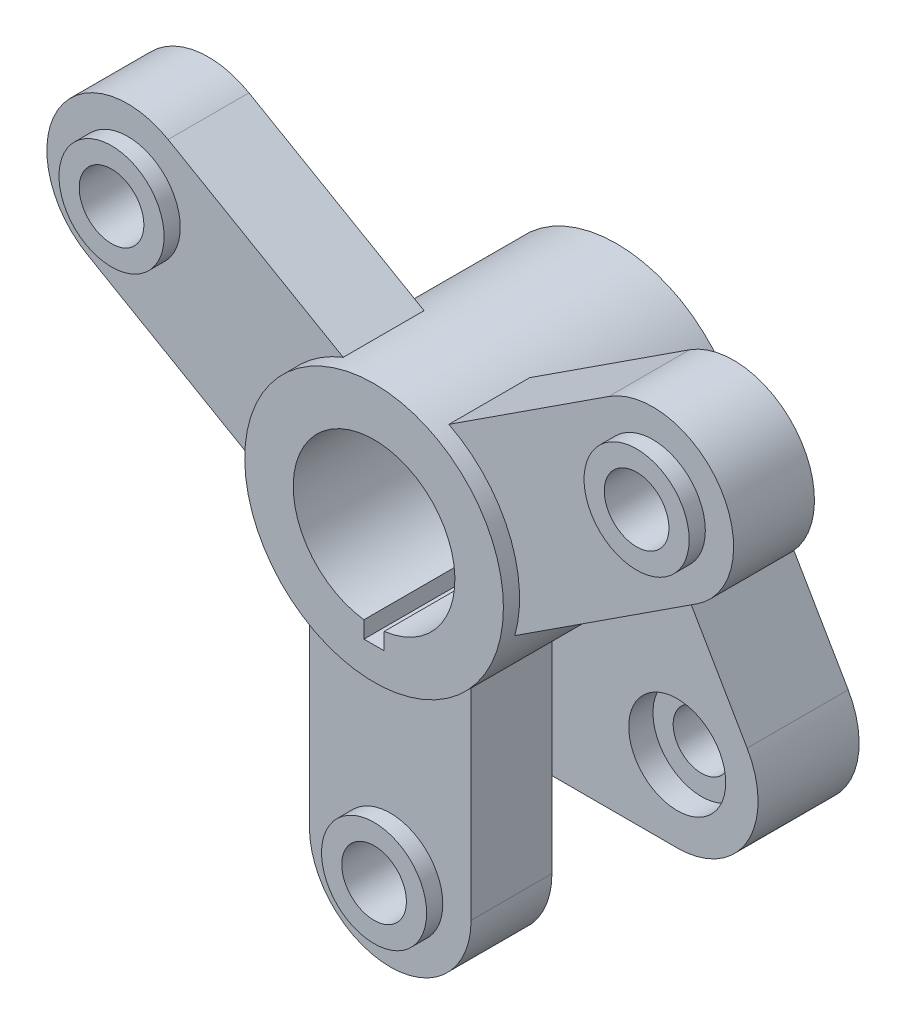
ISO-10303-21;
HEADER;
FILE_DESCRIPTION(('STEP AP214'),'2;1');
FILE_NAME('part.step','',(''),(''),'','','');
FILE_SCHEMA(('AUTOMOTIVE_DESIGN { 1 0 10303 214 1 1 1 1 }'));
ENDSEC;
DATA;
#1=APPLICATION_CONTEXT('core data for automotive mechanical design processes');
#2=APPLICATION_PROTOCOL_DEFINITION('international standard','automotive_design',2000,#1);
#3=PRODUCT_CONTEXT('',#1,'mechanical');
#4=PRODUCT('Part','Part','',(#3));
#5=PRODUCT_RELATED_PRODUCT_CATEGORY('part','',(#4));
#6=PRODUCT_DEFINITION_FORMATION('','',#4);
#7=PRODUCT_DEFINITION_CONTEXT('part definition',#1,'design');
#8=PRODUCT_DEFINITION('design','',#6,#7);
#9=PRODUCT_DEFINITION_SHAPE('','',#8);
#10=(LENGTH_UNIT() NAMED_UNIT(*) SI_UNIT(.MILLI.,.METRE.));
#11=(NAMED_UNIT(*) PLANE_ANGLE_UNIT() SI_UNIT($,.RADIAN.));
#12=(NAMED_UNIT(*) SI_UNIT($,.STERADIAN.) SOLID_ANGLE_UNIT());
#13=UNCERTAINTY_MEASURE_WITH_UNIT(LENGTH_MEASURE(1.E-05),#10,'distance_accuracy_value','');
#14=(GEOMETRIC_REPRESENTATION_CONTEXT(3) GLOBAL_UNCERTAINTY_ASSIGNED_CONTEXT((#13)) GLOBAL_UNIT_ASSIGNED_CONTEXT((#10,
#11,#12)) REPRESENTATION_CONTEXT('',''));
#15=CARTESIAN_POINT('',(0.,0.,0.));
#16=DIRECTION('',(0.,0.,1.));
#17=DIRECTION('',(1.,0.,0.));
#18=AXIS2_PLACEMENT_3D('',#15,#16,#17);
#19=CARTESIAN_POINT('',(0.,0.,56.));
#20=DIRECTION('',(0.,0.,1.));
#21=DIRECTION('',(1.,0.,0.));
#22=AXIS2_PLACEMENT_3D('',#19,#20,#21);
#23=PLANE('',#22);
#24=CARTESIAN_POINT('',(-64.9519052838331,37.4999999999997,56.));
#25=DIRECTION('',(0.,0.,1.));
#26=DIRECTION('',(1.,0.,0.));
#27=AXIS2_PLACEMENT_3D('',#24,#25,#26);
#28=CIRCLE('',#27,13.);
#29=CARTESIAN_POINT('',(-51.9519052838331,37.4999999999997,56.));
#30=VERTEX_POINT('',#29);
#31=EDGE_CURVE('E421',#30,#30,#28,.T.);
#32=ORIENTED_EDGE('',*,*,#31,.F.);
#33=EDGE_LOOP('',(#32));
#34=FACE_BOUND('',#33,.T.);
#35=CARTESIAN_POINT('',(0.,0.,56.));
#36=DIRECTION('',(0.,0.,1.));
#37=DIRECTION('',(1.,0.,0.));
#38=AXIS2_PLACEMENT_3D('',#35,#36,#37);
#39=CIRCLE('',#38,32.);
#40=CARTESIAN_POINT('',(-11.633307652784,29.8105040724855,56.));
#41=VERTEX_POINT('',#40);
#42=CARTESIAN_POINT('',(-31.6333076527839,-4.83051207889206,56.));
#43=VERTEX_POINT('',#42);
#44=EDGE_CURVE('E11',#41,#43,#39,.T.);
#45=ORIENTED_EDGE('',*,*,#44,.F.);
#46=DIRECTION('',(0.866025403784442,-0.499999999999995,0.));
#47=VECTOR('',#46,1.);
#48=CARTESIAN_POINT('',(9.99999999999993,17.3205080756889,56.));
#49=LINE('',#48,#47);
#50=CARTESIAN_POINT('',(-54.9519052838332,54.8205080756885,56.));
#51=VERTEX_POINT('',#50);
#52=EDGE_CURVE('E290',#51,#41,#49,.T.);
#53=ORIENTED_EDGE('',*,*,#52,.F.);
#54=CARTESIAN_POINT('',(-64.9519052838331,37.4999999999997,56.));
#55=DIRECTION('',(0.,0.,1.));
#56=DIRECTION('',(1.,0.,0.));
#57=AXIS2_PLACEMENT_3D('',#54,#55,#56);
#58=CIRCLE('',#57,20.);
#59=CARTESIAN_POINT('',(-74.951905283833,20.1794919243108,56.));
#60=VERTEX_POINT('',#59);
#61=EDGE_CURVE('E309',#51,#60,#58,.T.);
#62=ORIENTED_EDGE('',*,*,#61,.T.);
#63=DIRECTION('',(0.866025403784442,-0.499999999999994,0.));
#64=VECTOR('',#63,1.);
#65=CARTESIAN_POINT('',(-9.99999999999984,-17.3205080756887,56.));
#66=LINE('',#65,#64);
#67=EDGE_CURVE('E299',#60,#43,#66,.T.);
#68=ORIENTED_EDGE('',*,*,#67,.T.);
#69=EDGE_LOOP('',(#45,#53,#62,#68));
#70=FACE_BOUND('',#69,.T.);
#71=ADVANCED_FACE('F50',(#34,#70),#23,.T.);
#72=CARTESIAN_POINT('',(0.,-75.,56.));
#73=DIRECTION('',(0.,0.,1.));
#74=DIRECTION('',(1.,0.,0.));
#75=AXIS2_PLACEMENT_3D('',#72,#73,#74);
#76=CIRCLE('',#75,13.);
#77=CARTESIAN_POINT('',(13.,-75.,56.));
#78=VERTEX_POINT('',#77);
#79=EDGE_CURVE('E414',#78,#78,#76,.T.);
#80=ORIENTED_EDGE('',*,*,#79,.F.);
#81=EDGE_LOOP('',(#80));
#82=FACE_BOUND('',#81,.T.);
#83=CARTESIAN_POINT('',(-20.,-24.9799919935936,56.));
#84=VERTEX_POINT('',#83);
#85=CARTESIAN_POINT('',(20.,-24.9799919935936,56.));
#86=VERTEX_POINT('',#85);
#87=EDGE_CURVE('E57',#84,#86,#39,.T.);
#88=ORIENTED_EDGE('',*,*,#87,.F.);
#89=DIRECTION('',(0.,1.,0.));
#90=VECTOR('',#89,1.);
#91=CARTESIAN_POINT('',(-20.,0.,56.));
#92=LINE('',#91,#90);
#93=CARTESIAN_POINT('',(-20.,-75.,56.));
#94=VERTEX_POINT('',#93);
#95=EDGE_CURVE('E238',#94,#84,#92,.T.);
#96=ORIENTED_EDGE('',*,*,#95,.F.);
#97=CARTESIAN_POINT('',(0.,-75.,56.));
#98=DIRECTION('',(0.,0.,1.));
#99=DIRECTION('',(1.,0.,0.));
#100=AXIS2_PLACEMENT_3D('',#97,#98,#99);
#101=CIRCLE('',#100,20.);
#102=CARTESIAN_POINT('',(20.,-75.,56.));
#103=VERTEX_POINT('',#102);
#104=EDGE_CURVE('E251',#94,#103,#101,.T.);
#105=ORIENTED_EDGE('',*,*,#104,.T.);
#106=DIRECTION('',(0.,1.,0.));
#107=VECTOR('',#106,1.);
#108=CARTESIAN_POINT('',(20.,0.,56.));
#109=LINE('',#108,#107);
#110=EDGE_CURVE('E243',#103,#86,#109,.T.);
#111=ORIENTED_EDGE('',*,*,#110,.T.);
#112=EDGE_LOOP('',(#88,#96,#105,#111));
#113=FACE_BOUND('',#112,.T.);
#114=ADVANCED_FACE('F436',(#82,#113),#23,.T.);
#115=CARTESIAN_POINT('',(0.,0.,25.));
#116=DIRECTION('',(0.,0.,-1.));
#117=DIRECTION('',(-1.,0.,0.));
#118=AXIS2_PLACEMENT_3D('',#115,#116,#117);
#119=CYLINDRICAL_SURFACE('',#118,32.);
#120=DIRECTION('',(0.,0.,1.));
#121=VECTOR('',#120,1.);
#122=CARTESIAN_POINT('',(-11.633307652784,29.8105040724855,36.));
#123=LINE('',#122,#121);
#124=CARTESIAN_POINT('',(-11.633307652784,29.8105040724855,36.));
#125=VERTEX_POINT('',#124);
#126=EDGE_CURVE('E313',#125,#41,#123,.T.);
#127=ORIENTED_EDGE('',*,*,#126,.T.);
#128=ORIENTED_EDGE('',*,*,#44,.T.);
#129=DIRECTION('',(0.,0.,1.));
#130=VECTOR('',#129,1.);
#131=CARTESIAN_POINT('',(-31.6333076527839,-4.83051207889206,36.));
#132=LINE('',#131,#130);
#133=CARTESIAN_POINT('',(-31.6333076527839,-4.83051207889206,36.));
#134=VERTEX_POINT('',#133);
#135=EDGE_CURVE('E319',#134,#43,#132,.T.);
#136=ORIENTED_EDGE('',*,*,#135,.F.);
#137=CARTESIAN_POINT('',(0.,0.,36.));
#138=DIRECTION('',(0.,0.,1.));
#139=DIRECTION('',(1.,0.,0.));
#140=AXIS2_PLACEMENT_3D('',#137,#138,#139);
#141=CIRCLE('',#140,32.);
#142=EDGE_CURVE('E304',#125,#134,#141,.T.);
#143=ORIENTED_EDGE('',*,*,#142,.F.);
#144=EDGE_LOOP('',(#127,#128,#136,#143));
#145=FACE_BOUND('',#144,.T.);
#146=DIRECTION('',(0.,0.,1.));
#147=VECTOR('',#146,1.);
#148=CARTESIAN_POINT('',(-20.,-24.9799919935936,36.));
#149=LINE('',#148,#147);
#150=CARTESIAN_POINT('',(-20.,-24.9799919935936,36.));
#151=VERTEX_POINT('',#150);
#152=EDGE_CURVE('E259',#151,#84,#149,.T.);
#153=ORIENTED_EDGE('',*,*,#152,.T.);
#154=ORIENTED_EDGE('',*,*,#87,.T.);
#155=DIRECTION('',(0.,0.,1.));
#156=VECTOR('',#155,1.);
#157=CARTESIAN_POINT('',(20.,-24.9799919935936,36.));
#158=LINE('',#157,#156);
#159=CARTESIAN_POINT('',(20.,-24.9799919935936,36.));
#160=VERTEX_POINT('',#159);
#161=EDGE_CURVE('E265',#160,#86,#158,.T.);
#162=ORIENTED_EDGE('',*,*,#161,.F.);
#163=CARTESIAN_POINT('',(0.,0.,36.));
#164=DIRECTION('',(0.,0.,1.));
#165=DIRECTION('',(1.,0.,0.));
#166=AXIS2_PLACEMENT_3D('',#163,#164,#165);
#167=CIRCLE('',#166,32.);
#168=EDGE_CURVE('E248',#151,#160,#167,.T.);
#169=ORIENTED_EDGE('',*,*,#168,.F.);
#170=EDGE_LOOP('',(#153,#154,#162,#169));
#171=FACE_BOUND('',#170,.T.);
#172=CARTESIAN_POINT('',(0.,0.,0.));
#173=DIRECTION('',(0.,0.,1.));
#174=DIRECTION('',(1.,0.,0.));
#175=AXIS2_PLACEMENT_3D('',#172,#173,#174);
#176=CIRCLE('',#175,32.);
#177=CARTESIAN_POINT('',(27.6744827586207,16.0662068965517,0.));
#178=VERTEX_POINT('',#177);
#179=CARTESIAN_POINT('',(-27.6744827586207,16.0662068965517,0.));
#180=VERTEX_POINT('',#179);
#181=EDGE_CURVE('E351',#178,#180,#176,.T.);
#182=ORIENTED_EDGE('',*,*,#181,.T.);
#183=DIRECTION('',(0.,0.,-1.));
#184=VECTOR('',#183,1.);
#185=CARTESIAN_POINT('',(-27.6744827586207,16.0662068965517,25.));
#186=LINE('',#185,#184);
#187=CARTESIAN_POINT('',(-27.6744827586207,16.0662068965517,25.));
#188=VERTEX_POINT('',#187);
#189=EDGE_CURVE('E365',#188,#180,#186,.T.);
#190=ORIENTED_EDGE('',*,*,#189,.F.);
#191=CARTESIAN_POINT('',(0.,0.,25.));
#192=DIRECTION('',(0.,0.,1.));
#193=DIRECTION('',(1.,0.,0.));
#194=AXIS2_PLACEMENT_3D('',#191,#192,#193);
#195=CIRCLE('',#194,32.);
#196=CARTESIAN_POINT('',(27.6744827586207,16.0662068965517,25.));
#197=VERTEX_POINT('',#196);
#198=EDGE_CURVE('E321',#188,#197,#195,.T.);
#199=ORIENTED_EDGE('',*,*,#198,.T.);
#200=DIRECTION('',(0.,0.,-1.));
#201=VECTOR('',#200,1.);
#202=CARTESIAN_POINT('',(27.6744827586207,16.0662068965517,25.));
#203=LINE('',#202,#201);
#204=EDGE_CURVE('E364',#197,#178,#203,.T.);
#205=ORIENTED_EDGE('',*,*,#204,.T.);
#206=EDGE_LOOP('',(#182,#190,#199,#205));
#207=FACE_BOUND('',#206,.T.);
#208=CARTESIAN_POINT('',(30.8276383277299,-8.58234904526002,56.));
#209=VERTEX_POINT('',#208);
#210=CARTESIAN_POINT('',(14.5071990180257,28.5226432269416,56.));
#211=VERTEX_POINT('',#210);
#212=EDGE_CURVE('E59',#209,#211,#39,.T.);
#213=ORIENTED_EDGE('',*,*,#212,.T.);
#214=DIRECTION('',(0.,0.,1.));
#215=VECTOR('',#214,1.);
#216=CARTESIAN_POINT('',(14.5071990180257,28.5226432269415,36.));
#217=LINE('',#216,#215);
#218=CARTESIAN_POINT('',(14.5071990180257,28.5226432269415,36.));
#219=VERTEX_POINT('',#218);
#220=EDGE_CURVE('E293',#219,#211,#217,.T.);
#221=ORIENTED_EDGE('',*,*,#220,.F.);
#222=CARTESIAN_POINT('',(0.,0.,36.));
#223=DIRECTION('',(0.,0.,1.));
#224=DIRECTION('',(1.,0.,0.));
#225=AXIS2_PLACEMENT_3D('',#222,#223,#224);
#226=CIRCLE('',#225,32.);
#227=CARTESIAN_POINT('',(30.8276383277299,-8.58234904526002,36.));
#228=VERTEX_POINT('',#227);
#229=EDGE_CURVE('E280',#228,#219,#226,.T.);
#230=ORIENTED_EDGE('',*,*,#229,.F.);
#231=DIRECTION('',(0.,0.,1.));
#232=VECTOR('',#231,1.);
#233=CARTESIAN_POINT('',(30.8276383277299,-8.58234904526002,36.));
#234=LINE('',#233,#232);
#235=EDGE_CURVE('E287',#228,#209,#234,.T.);
#236=ORIENTED_EDGE('',*,*,#235,.T.);
#237=EDGE_LOOP('',(#213,#221,#230,#236));
#238=FACE_BOUND('',#237,.T.);
#239=CARTESIAN_POINT('',(0.,0.,60.));
#240=DIRECTION('',(0.,0.,1.));
#241=DIRECTION('',(1.,0.,0.));
#242=AXIS2_PLACEMENT_3D('',#239,#240,#241);
#243=CIRCLE('',#242,32.);
#244=CARTESIAN_POINT('',(32.,0.,60.));
#245=VERTEX_POINT('',#244);
#246=EDGE_CURVE('E236',#245,#245,#243,.T.);
#247=ORIENTED_EDGE('',*,*,#246,.F.);
#248=EDGE_LOOP('',(#247));
#249=FACE_BOUND('',#248,.T.);
#250=ADVANCED_FACE('F446',(#145,#171,#207,#238,#249),#119,.T.);
#251=CARTESIAN_POINT('',(0.,-65.,25.));
#252=DIRECTION('',(0.,1.,0.));
#253=DIRECTION('',(0.,0.,1.));
#254=AXIS2_PLACEMENT_3D('',#251,#252,#253);
#255=PLANE('',#254);
#256=DIRECTION('',(1.,0.,0.));
#257=VECTOR('',#256,1.);
#258=CARTESIAN_POINT('',(0.,-65.,0.));
#259=LINE('',#258,#257);
#260=CARTESIAN_POINT('',(-40.,-65.,0.));
#261=VERTEX_POINT('',#260);
#262=CARTESIAN_POINT('',(40.,-65.,0.));
#263=VERTEX_POINT('',#262);
#264=EDGE_CURVE('E320',#261,#263,#259,.T.);
#265=ORIENTED_EDGE('',*,*,#264,.T.);
#266=DIRECTION('',(0.,0.,-1.));
#267=VECTOR('',#266,1.);
#268=CARTESIAN_POINT('',(40.,-65.,25.));
#269=LINE('',#268,#267);
#270=CARTESIAN_POINT('',(40.,-65.,25.));
#271=VERTEX_POINT('',#270);
#272=EDGE_CURVE('E330',#271,#263,#269,.T.);
#273=ORIENTED_EDGE('',*,*,#272,.F.);
#274=DIRECTION('',(1.,0.,0.));
#275=VECTOR('',#274,1.);
#276=CARTESIAN_POINT('',(0.,-65.,25.));
#277=LINE('',#276,#275);
#278=CARTESIAN_POINT('',(-40.,-65.,25.));
#279=VERTEX_POINT('',#278);
#280=EDGE_CURVE('E329',#279,#271,#277,.T.);
#281=ORIENTED_EDGE('',*,*,#280,.F.);
#282=DIRECTION('',(0.,0.,-1.));
#283=VECTOR('',#282,1.);
#284=CARTESIAN_POINT('',(-40.,-65.,25.));
#285=LINE('',#284,#283);
#286=EDGE_CURVE('E345',#279,#261,#285,.T.);
#287=ORIENTED_EDGE('',*,*,#286,.T.);
#288=EDGE_LOOP('',(#265,#273,#281,#287));
#289=FACE_BOUND('',#288,.T.);
#290=ADVANCED_FACE('F47',(#289),#255,.F.);
#291=CARTESIAN_POINT('',(40.,-45.,25.));
#292=DIRECTION('',(0.,0.,-1.));
#293=DIRECTION('',(-1.,0.,0.));
#294=AXIS2_PLACEMENT_3D('',#291,#292,#293);
#295=CYLINDRICAL_SURFACE('',#294,20.);
#296=CARTESIAN_POINT('',(40.,-45.,0.));
#297=DIRECTION('',(0.,0.,1.));
#298=DIRECTION('',(1.,0.,0.));
#299=AXIS2_PLACEMENT_3D('',#296,#297,#298);
#300=CIRCLE('',#299,20.);
#301=CARTESIAN_POINT('',(57.2965517241379,-34.9586206896552,0.));
#302=VERTEX_POINT('',#301);
#303=EDGE_CURVE('E343',#263,#302,#300,.T.);
#304=ORIENTED_EDGE('',*,*,#303,.T.);
#305=DIRECTION('',(0.,0.,-1.));
#306=VECTOR('',#305,1.);
#307=CARTESIAN_POINT('',(57.2965517241379,-34.9586206896552,25.));
#308=LINE('',#307,#306);
#309=CARTESIAN_POINT('',(57.2965517241379,-34.9586206896552,25.));
#310=VERTEX_POINT('',#309);
#311=EDGE_CURVE('E366',#310,#302,#308,.T.);
#312=ORIENTED_EDGE('',*,*,#311,.F.);
#313=CARTESIAN_POINT('',(40.,-45.,25.));
#314=DIRECTION('',(0.,0.,1.));
#315=DIRECTION('',(1.,0.,0.));
#316=AXIS2_PLACEMENT_3D('',#313,#314,#315);
#317=CIRCLE('',#316,20.);
#318=EDGE_CURVE('E331',#271,#310,#317,.T.);
#319=ORIENTED_EDGE('',*,*,#318,.F.);
#320=ORIENTED_EDGE('',*,*,#272,.T.);
#321=EDGE_LOOP('',(#304,#312,#319,#320));
#322=FACE_BOUND('',#321,.T.);
#323=ADVANCED_FACE('F492',(#322),#295,.T.);
#324=CARTESIAN_POINT('',(27.6744827586207,16.0662068965517,25.));
#325=DIRECTION('',(0.864827586206897,0.502068965517242,0.));
#326=DIRECTION('',(-0.502068965517242,0.864827586206897,0.));
#327=AXIS2_PLACEMENT_3D('',#324,#325,#326);
#328=PLANE('',#327);
#329=DIRECTION('',(0.502068965517242,-0.864827586206897,0.));
#330=VECTOR('',#329,1.);
#331=CARTESIAN_POINT('',(27.6744827586207,16.0662068965517,0.));
#332=LINE('',#331,#330);
#333=EDGE_CURVE('E349',#178,#302,#332,.T.);
#334=ORIENTED_EDGE('',*,*,#333,.F.);
#335=ORIENTED_EDGE('',*,*,#204,.F.);
#336=DIRECTION('',(0.502068965517242,-0.864827586206897,0.));
#337=VECTOR('',#336,1.);
#338=CARTESIAN_POINT('',(27.6744827586207,16.0662068965517,25.));
#339=LINE('',#338,#337);
#340=EDGE_CURVE('E333',#197,#310,#339,.T.);
#341=ORIENTED_EDGE('',*,*,#340,.T.);
#342=ORIENTED_EDGE('',*,*,#311,.T.);
#343=EDGE_LOOP('',(#334,#335,#341,#342));
#344=FACE_BOUND('',#343,.T.);
#345=ADVANCED_FACE('F489',(#344),#328,.T.);
#346=CARTESIAN_POINT('',(-27.6744827586207,16.0662068965517,25.));
#347=DIRECTION('',(-0.864827586206896,0.502068965517242,0.));
#348=DIRECTION('',(-0.502068965517242,-0.864827586206896,0.));
#349=AXIS2_PLACEMENT_3D('',#346,#347,#348);
#350=PLANE('',#349);
#351=DIRECTION('',(0.502068965517242,0.864827586206896,0.));
#352=VECTOR('',#351,1.);
#353=CARTESIAN_POINT('',(-27.6744827586207,16.0662068965517,0.));
#354=LINE('',#353,#352);
#355=CARTESIAN_POINT('',(-57.2965517241379,-34.9586206896552,0.));
#356=VERTEX_POINT('',#355);
#357=EDGE_CURVE('E353',#356,#180,#354,.T.);
#358=ORIENTED_EDGE('',*,*,#357,.F.);
#359=DIRECTION('',(0.,0.,-1.));
#360=VECTOR('',#359,1.);
#361=CARTESIAN_POINT('',(-57.2965517241379,-34.9586206896552,25.));
#362=LINE('',#361,#360);
#363=CARTESIAN_POINT('',(-57.2965517241379,-34.9586206896552,25.));
#364=VERTEX_POINT('',#363);
#365=EDGE_CURVE('E359',#364,#356,#362,.T.);
#366=ORIENTED_EDGE('',*,*,#365,.F.);
#367=DIRECTION('',(0.502068965517242,0.864827586206896,0.));
#368=VECTOR('',#367,1.);
#369=CARTESIAN_POINT('',(-27.6744827586207,16.0662068965517,25.));
#370=LINE('',#369,#368);
#371=EDGE_CURVE('E340',#364,#188,#370,.T.);
#372=ORIENTED_EDGE('',*,*,#371,.T.);
#373=ORIENTED_EDGE('',*,*,#189,.T.);
#374=EDGE_LOOP('',(#358,#366,#372,#373));
#375=FACE_BOUND('',#374,.T.);
#376=ADVANCED_FACE('F487',(#375),#350,.T.);
#377=CARTESIAN_POINT('',(-40.,-45.,25.));
#378=DIRECTION('',(0.,0.,-1.));
#379=DIRECTION('',(-1.,0.,0.));
#380=AXIS2_PLACEMENT_3D('',#377,#378,#379);
#381=CYLINDRICAL_SURFACE('',#380,20.);
#382=CARTESIAN_POINT('',(-40.,-45.,0.));
#383=DIRECTION('',(0.,0.,1.));
#384=DIRECTION('',(1.,0.,0.));
#385=AXIS2_PLACEMENT_3D('',#382,#383,#384);
#386=CIRCLE('',#385,20.);
#387=EDGE_CURVE('E332',#356,#261,#386,.T.);
#388=ORIENTED_EDGE('',*,*,#387,.T.);
#389=ORIENTED_EDGE('',*,*,#286,.F.);
#390=CARTESIAN_POINT('',(-40.,-45.,25.));
#391=DIRECTION('',(0.,0.,1.));
#392=DIRECTION('',(1.,0.,0.));
#393=AXIS2_PLACEMENT_3D('',#390,#391,#392);
#394=CIRCLE('',#393,20.);
#395=EDGE_CURVE('E338',#364,#279,#394,.T.);
#396=ORIENTED_EDGE('',*,*,#395,.F.);
#397=ORIENTED_EDGE('',*,*,#365,.T.);
#398=EDGE_LOOP('',(#388,#389,#396,#397));
#399=FACE_BOUND('',#398,.T.);
#400=ADVANCED_FACE('F478',(#399),#381,.T.);
#401=CARTESIAN_POINT('',(0.,0.,25.));
#402=DIRECTION('',(0.,0.,1.));
#403=DIRECTION('',(1.,0.,0.));
#404=AXIS2_PLACEMENT_3D('',#401,#402,#403);
#405=PLANE('',#404);
#406=CARTESIAN_POINT('',(-40.,-45.,25.));
#407=DIRECTION('',(0.,0.,1.));
#408=DIRECTION('',(1.,0.,0.));
#409=AXIS2_PLACEMENT_3D('',#406,#407,#408);
#410=CIRCLE('',#409,12.);
#411=CARTESIAN_POINT('',(-28.,-45.,25.));
#412=VERTEX_POINT('',#411);
#413=EDGE_CURVE('E389',#412,#412,#410,.T.);
#414=ORIENTED_EDGE('',*,*,#413,.F.);
#415=EDGE_LOOP('',(#414));
#416=FACE_BOUND('',#415,.T.);
#417=CARTESIAN_POINT('',(40.,-45.,25.));
#418=DIRECTION('',(0.,0.,1.));
#419=DIRECTION('',(1.,0.,0.));
#420=AXIS2_PLACEMENT_3D('',#417,#418,#419);
#421=CIRCLE('',#420,12.);
#422=CARTESIAN_POINT('',(52.,-45.,25.));
#423=VERTEX_POINT('',#422);
#424=EDGE_CURVE('E374',#423,#423,#421,.T.);
#425=ORIENTED_EDGE('',*,*,#424,.F.);
#426=EDGE_LOOP('',(#425));
#427=FACE_BOUND('',#426,.T.);
#428=ORIENTED_EDGE('',*,*,#198,.F.);
#429=ORIENTED_EDGE('',*,*,#371,.F.);
#430=ORIENTED_EDGE('',*,*,#395,.T.);
#431=ORIENTED_EDGE('',*,*,#280,.T.);
#432=ORIENTED_EDGE('',*,*,#318,.T.);
#433=ORIENTED_EDGE('',*,*,#340,.F.);
#434=EDGE_LOOP('',(#428,#429,#430,#431,#432,#433));
#435=FACE_BOUND('',#434,.T.);
#436=ADVANCED_FACE('F480',(#416,#427,#435),#405,.T.);
#437=CARTESIAN_POINT('',(0.,0.,0.));
#438=DIRECTION('',(0.,0.,1.));
#439=DIRECTION('',(1.,0.,0.));
#440=AXIS2_PLACEMENT_3D('',#437,#438,#439);
#441=PLANE('',#440);
#442=CARTESIAN_POINT('',(-40.,-45.,0.));
#443=DIRECTION('',(0.,0.,1.));
#444=DIRECTION('',(1.,0.,0.));
#445=AXIS2_PLACEMENT_3D('',#442,#443,#444);
#446=CIRCLE('',#445,7.);
#447=CARTESIAN_POINT('',(-33.,-45.,0.));
#448=VERTEX_POINT('',#447);
#449=EDGE_CURVE('E51',#448,#448,#446,.T.);
#450=ORIENTED_EDGE('',*,*,#449,.T.);
#451=EDGE_LOOP('',(#450));
#452=FACE_BOUND('',#451,.T.);
#453=CARTESIAN_POINT('',(40.,-45.,0.));
#454=DIRECTION('',(0.,0.,1.));
#455=DIRECTION('',(1.,0.,0.));
#456=AXIS2_PLACEMENT_3D('',#453,#454,#455);
#457=CIRCLE('',#456,6.99999999999999);
#458=CARTESIAN_POINT('',(47.,-45.,0.));
#459=VERTEX_POINT('',#458);
#460=EDGE_CURVE('E367',#459,#459,#457,.T.);
#461=ORIENTED_EDGE('',*,*,#460,.T.);
#462=EDGE_LOOP('',(#461));
#463=FACE_BOUND('',#462,.T.);
#464=DIRECTION('',(0.,1.,0.));
#465=VECTOR('',#464,1.);
#466=CARTESIAN_POINT('',(2.5,0.,0.));
#467=LINE('',#466,#465);
#468=CARTESIAN_POINT('',(2.5,-24.,0.));
#469=VERTEX_POINT('',#468);
#470=CARTESIAN_POINT('',(2.5,-19.8431348329844,0.));
#471=VERTEX_POINT('',#470);
#472=EDGE_CURVE('E229',#469,#471,#467,.T.);
#473=ORIENTED_EDGE('',*,*,#472,.T.);
#474=CARTESIAN_POINT('',(0.,0.,0.));
#475=DIRECTION('',(0.,0.,1.));
#476=DIRECTION('',(1.,0.,0.));
#477=AXIS2_PLACEMENT_3D('',#474,#475,#476);
#478=CIRCLE('',#477,20.);
#479=CARTESIAN_POINT('',(-2.5,-19.8431348329844,0.));
#480=VERTEX_POINT('',#479);
#481=EDGE_CURVE('E231',#471,#480,#478,.T.);
#482=ORIENTED_EDGE('',*,*,#481,.T.);
#483=DIRECTION('',(0.,-1.,0.));
#484=VECTOR('',#483,1.);
#485=CARTESIAN_POINT('',(-2.5,0.,0.));
#486=LINE('',#485,#484);
#487=CARTESIAN_POINT('',(-2.5,-24.,0.));
#488=VERTEX_POINT('',#487);
#489=EDGE_CURVE('E225',#480,#488,#486,.T.);
#490=ORIENTED_EDGE('',*,*,#489,.T.);
#491=DIRECTION('',(1.,0.,0.));
#492=VECTOR('',#491,1.);
#493=CARTESIAN_POINT('',(0.,-24.,0.));
#494=LINE('',#493,#492);
#495=EDGE_CURVE('E205',#488,#469,#494,.T.);
#496=ORIENTED_EDGE('',*,*,#495,.T.);
#497=EDGE_LOOP('',(#473,#482,#490,#496));
#498=FACE_BOUND('',#497,.T.);
#499=ORIENTED_EDGE('',*,*,#264,.F.);
#500=ORIENTED_EDGE('',*,*,#387,.F.);
#501=ORIENTED_EDGE('',*,*,#357,.T.);
#502=ORIENTED_EDGE('',*,*,#181,.F.);
#503=ORIENTED_EDGE('',*,*,#333,.T.);
#504=ORIENTED_EDGE('',*,*,#303,.F.);
#505=EDGE_LOOP('',(#499,#500,#501,#502,#503,#504));
#506=FACE_BOUND('',#505,.T.);
#507=ADVANCED_FACE('F473',(#452,#463,#498,#506),#441,.F.);
#508=CARTESIAN_POINT('',(64.951905283833,37.4999999999998,56.));
#509=DIRECTION('',(0.,0.,1.));
#510=DIRECTION('',(1.,0.,0.));
#511=AXIS2_PLACEMENT_3D('',#508,#509,#510);
#512=CIRCLE('',#511,13.);
#513=CARTESIAN_POINT('',(77.951905283833,37.4999999999998,56.));
#514=VERTEX_POINT('',#513);
#515=EDGE_CURVE('E417',#514,#514,#512,.T.);
#516=ORIENTED_EDGE('',*,*,#515,.F.);
#517=EDGE_LOOP('',(#516));
#518=FACE_BOUND('',#517,.T.);
#519=ORIENTED_EDGE('',*,*,#212,.F.);
#520=DIRECTION('',(-0.83803643049516,-0.545614278738132,0.));
#521=VECTOR('',#520,1.);
#522=CARTESIAN_POINT('',(13.1014650998701,-20.1231996199676,56.));
#523=LINE('',#522,#521);
#524=CARTESIAN_POINT('',(75.8641908585956,20.7392713900967,56.));
#525=VERTEX_POINT('',#524);
#526=EDGE_CURVE('E262',#525,#209,#523,.T.);
#527=ORIENTED_EDGE('',*,*,#526,.F.);
#528=CARTESIAN_POINT('',(64.951905283833,37.4999999999998,56.));
#529=DIRECTION('',(0.,0.,1.));
#530=DIRECTION('',(1.,0.,0.));
#531=AXIS2_PLACEMENT_3D('',#528,#529,#530);
#532=CIRCLE('',#531,20.);
#533=CARTESIAN_POINT('',(54.0396197090703,54.260728609903,56.));
#534=VERTEX_POINT('',#533);
#535=EDGE_CURVE('E285',#525,#534,#532,.T.);
#536=ORIENTED_EDGE('',*,*,#535,.T.);
#537=DIRECTION('',(-0.83803643049516,-0.545614278738131,0.));
#538=VECTOR('',#537,1.);
#539=CARTESIAN_POINT('',(-8.72310604965517,13.3982575998388,56.));
#540=LINE('',#539,#538);
#541=EDGE_CURVE('E272',#534,#211,#540,.T.);
#542=ORIENTED_EDGE('',*,*,#541,.T.);
#543=EDGE_LOOP('',(#519,#527,#536,#542));
#544=FACE_BOUND('',#543,.T.);
#545=ADVANCED_FACE('F438',(#518,#544),#23,.T.);
#546=CARTESIAN_POINT('',(9.99999999999993,17.3205080756889,36.));
#547=DIRECTION('',(-0.499999999999995,-0.866025403784442,0.));
#548=DIRECTION('',(0.866025403784442,-0.499999999999995,0.));
#549=AXIS2_PLACEMENT_3D('',#546,#547,#548);
#550=PLANE('',#549);
#551=ORIENTED_EDGE('',*,*,#52,.T.);
#552=ORIENTED_EDGE('',*,*,#126,.F.);
#553=DIRECTION('',(0.866025403784442,-0.499999999999995,0.));
#554=VECTOR('',#553,1.);
#555=CARTESIAN_POINT('',(9.99999999999993,17.3205080756889,36.));
#556=LINE('',#555,#554);
#557=CARTESIAN_POINT('',(-54.9519052838332,54.8205080756885,36.));
#558=VERTEX_POINT('',#557);
#559=EDGE_CURVE('E298',#558,#125,#556,.T.);
#560=ORIENTED_EDGE('',*,*,#559,.F.);
#561=DIRECTION('',(0.,0.,1.));
#562=VECTOR('',#561,1.);
#563=CARTESIAN_POINT('',(-54.9519052838332,54.8205080756885,36.));
#564=LINE('',#563,#562);
#565=EDGE_CURVE('E310',#558,#51,#564,.T.);
#566=ORIENTED_EDGE('',*,*,#565,.T.);
#567=EDGE_LOOP('',(#551,#552,#560,#566));
#568=FACE_BOUND('',#567,.T.);
#569=ADVANCED_FACE('F447',(#568),#550,.F.);
#570=CARTESIAN_POINT('',(-9.99999999999984,-17.3205080756887,36.));
#571=DIRECTION('',(-0.499999999999994,-0.866025403784442,0.));
#572=DIRECTION('',(0.866025403784442,-0.499999999999994,0.));
#573=AXIS2_PLACEMENT_3D('',#570,#571,#572);
#574=PLANE('',#573);
#575=ORIENTED_EDGE('',*,*,#67,.F.);
#576=DIRECTION('',(0.,0.,1.));
#577=VECTOR('',#576,1.);
#578=CARTESIAN_POINT('',(-74.951905283833,20.1794919243108,36.));
#579=LINE('',#578,#577);
#580=CARTESIAN_POINT('',(-74.951905283833,20.1794919243108,36.));
#581=VERTEX_POINT('',#580);
#582=EDGE_CURVE('E322',#581,#60,#579,.T.);
#583=ORIENTED_EDGE('',*,*,#582,.F.);
#584=DIRECTION('',(0.866025403784442,-0.499999999999994,0.));
#585=VECTOR('',#584,1.);
#586=CARTESIAN_POINT('',(-9.99999999999984,-17.3205080756887,36.));
#587=LINE('',#586,#585);
#588=EDGE_CURVE('E305',#581,#134,#587,.T.);
#589=ORIENTED_EDGE('',*,*,#588,.T.);
#590=ORIENTED_EDGE('',*,*,#135,.T.);
#591=EDGE_LOOP('',(#575,#583,#589,#590));
#592=FACE_BOUND('',#591,.T.);
#593=ADVANCED_FACE('F457',(#592),#574,.T.);
#594=CARTESIAN_POINT('',(-64.9519052838331,37.4999999999997,36.));
#595=DIRECTION('',(0.,0.,1.));
#596=DIRECTION('',(1.,0.,0.));
#597=AXIS2_PLACEMENT_3D('',#594,#595,#596);
#598=CYLINDRICAL_SURFACE('',#597,20.);
#599=ORIENTED_EDGE('',*,*,#61,.F.);
#600=ORIENTED_EDGE('',*,*,#565,.F.);
#601=CARTESIAN_POINT('',(-64.9519052838331,37.4999999999997,36.));
#602=DIRECTION('',(0.,0.,1.));
#603=DIRECTION('',(1.,0.,0.));
#604=AXIS2_PLACEMENT_3D('',#601,#602,#603);
#605=CIRCLE('',#604,20.);
#606=EDGE_CURVE('E296',#558,#581,#605,.T.);
#607=ORIENTED_EDGE('',*,*,#606,.T.);
#608=ORIENTED_EDGE('',*,*,#582,.T.);
#609=EDGE_LOOP('',(#599,#600,#607,#608));
#610=FACE_BOUND('',#609,.T.);
#611=ADVANCED_FACE('F459',(#610),#598,.T.);
#612=CARTESIAN_POINT('',(0.,0.,36.));
#613=DIRECTION('',(0.,0.,1.));
#614=DIRECTION('',(1.,0.,0.));
#615=AXIS2_PLACEMENT_3D('',#612,#613,#614);
#616=PLANE('',#615);
#617=CARTESIAN_POINT('',(-64.9519052838331,37.4999999999997,36.));
#618=DIRECTION('',(0.,0.,1.));
#619=DIRECTION('',(1.,0.,0.));
#620=AXIS2_PLACEMENT_3D('',#617,#618,#619);
#621=CIRCLE('',#620,8.);
#622=CARTESIAN_POINT('',(-56.9519052838331,37.4999999999997,36.));
#623=VERTEX_POINT('',#622);
#624=EDGE_CURVE('E408',#623,#623,#621,.T.);
#625=ORIENTED_EDGE('',*,*,#624,.T.);
#626=EDGE_LOOP('',(#625));
#627=FACE_BOUND('',#626,.T.);
#628=ORIENTED_EDGE('',*,*,#559,.T.);
#629=ORIENTED_EDGE('',*,*,#142,.T.);
#630=ORIENTED_EDGE('',*,*,#588,.F.);
#631=ORIENTED_EDGE('',*,*,#606,.F.);
#632=EDGE_LOOP('',(#628,#629,#630,#631));
#633=FACE_BOUND('',#632,.T.);
#634=ADVANCED_FACE('F454',(#627,#633),#616,.F.);
#635=CARTESIAN_POINT('',(13.1014650998701,-20.1231996199676,36.));
#636=DIRECTION('',(-0.545614278738132,0.83803643049516,0.));
#637=DIRECTION('',(-0.83803643049516,-0.545614278738132,0.));
#638=AXIS2_PLACEMENT_3D('',#635,#636,#637);
#639=PLANE('',#638);
#640=ORIENTED_EDGE('',*,*,#526,.T.);
#641=ORIENTED_EDGE('',*,*,#235,.F.);
#642=DIRECTION('',(-0.83803643049516,-0.545614278738132,0.));
#643=VECTOR('',#642,1.);
#644=CARTESIAN_POINT('',(13.1014650998701,-20.1231996199676,36.));
#645=LINE('',#644,#643);
#646=CARTESIAN_POINT('',(75.8641908585956,20.7392713900967,36.));
#647=VERTEX_POINT('',#646);
#648=EDGE_CURVE('E269',#647,#228,#645,.T.);
#649=ORIENTED_EDGE('',*,*,#648,.F.);
#650=DIRECTION('',(0.,0.,1.));
#651=VECTOR('',#650,1.);
#652=CARTESIAN_POINT('',(75.8641908585956,20.7392713900967,36.));
#653=LINE('',#652,#651);
#654=EDGE_CURVE('E276',#647,#525,#653,.T.);
#655=ORIENTED_EDGE('',*,*,#654,.T.);
#656=EDGE_LOOP('',(#640,#641,#649,#655));
#657=FACE_BOUND('',#656,.T.);
#658=ADVANCED_FACE('F467',(#657),#639,.F.);
#659=CARTESIAN_POINT('',(-8.72310604965517,13.3982575998388,36.));
#660=DIRECTION('',(-0.545614278738131,0.83803643049516,0.));
#661=DIRECTION('',(-0.83803643049516,-0.545614278738131,0.));
#662=AXIS2_PLACEMENT_3D('',#659,#660,#661);
#663=PLANE('',#662);
#664=ORIENTED_EDGE('',*,*,#541,.F.);
#665=DIRECTION('',(0.,0.,1.));
#666=VECTOR('',#665,1.);
#667=CARTESIAN_POINT('',(54.0396197090703,54.260728609903,36.));
#668=LINE('',#667,#666);
#669=CARTESIAN_POINT('',(54.0396197090703,54.260728609903,36.));
#670=VERTEX_POINT('',#669);
#671=EDGE_CURVE('E291',#670,#534,#668,.T.);
#672=ORIENTED_EDGE('',*,*,#671,.F.);
#673=DIRECTION('',(-0.83803643049516,-0.545614278738131,0.));
#674=VECTOR('',#673,1.);
#675=CARTESIAN_POINT('',(-8.72310604965517,13.3982575998388,36.));
#676=LINE('',#675,#674);
#677=EDGE_CURVE('E274',#670,#219,#676,.T.);
#678=ORIENTED_EDGE('',*,*,#677,.T.);
#679=ORIENTED_EDGE('',*,*,#220,.T.);
#680=EDGE_LOOP('',(#664,#672,#678,#679));
#681=FACE_BOUND('',#680,.T.);
#682=ADVANCED_FACE('F554',(#681),#663,.T.);
#683=CARTESIAN_POINT('',(64.951905283833,37.4999999999998,36.));
#684=DIRECTION('',(0.,0.,1.));
#685=DIRECTION('',(1.,0.,0.));
#686=AXIS2_PLACEMENT_3D('',#683,#684,#685);
#687=CYLINDRICAL_SURFACE('',#686,20.);
#688=ORIENTED_EDGE('',*,*,#535,.F.);
#689=ORIENTED_EDGE('',*,*,#654,.F.);
#690=CARTESIAN_POINT('',(64.951905283833,37.4999999999998,36.));
#691=DIRECTION('',(0.,0.,1.));
#692=DIRECTION('',(1.,0.,0.));
#693=AXIS2_PLACEMENT_3D('',#690,#691,#692);
#694=CIRCLE('',#693,20.);
#695=EDGE_CURVE('E270',#647,#670,#694,.T.);
#696=ORIENTED_EDGE('',*,*,#695,.T.);
#697=ORIENTED_EDGE('',*,*,#671,.T.);
#698=EDGE_LOOP('',(#688,#689,#696,#697));
#699=FACE_BOUND('',#698,.T.);
#700=ADVANCED_FACE('F551',(#699),#687,.T.);
#701=CARTESIAN_POINT('',(0.,0.,36.));
#702=DIRECTION('',(0.,0.,1.));
#703=DIRECTION('',(1.,0.,0.));
#704=AXIS2_PLACEMENT_3D('',#701,#702,#703);
#705=PLANE('',#704);
#706=CARTESIAN_POINT('',(64.951905283833,37.4999999999998,36.));
#707=DIRECTION('',(0.,0.,1.));
#708=DIRECTION('',(1.,0.,0.));
#709=AXIS2_PLACEMENT_3D('',#706,#707,#708);
#710=CIRCLE('',#709,8.);
#711=CARTESIAN_POINT('',(72.951905283833,37.4999999999998,36.));
#712=VERTEX_POINT('',#711);
#713=EDGE_CURVE('E410',#712,#712,#710,.T.);
#714=ORIENTED_EDGE('',*,*,#713,.T.);
#715=EDGE_LOOP('',(#714));
#716=FACE_BOUND('',#715,.T.);
#717=ORIENTED_EDGE('',*,*,#648,.T.);
#718=ORIENTED_EDGE('',*,*,#229,.T.);
#719=ORIENTED_EDGE('',*,*,#677,.F.);
#720=ORIENTED_EDGE('',*,*,#695,.F.);
#721=EDGE_LOOP('',(#717,#718,#719,#720));
#722=FACE_BOUND('',#721,.T.);
#723=ADVANCED_FACE('F548',(#716,#722),#705,.F.);
#724=CARTESIAN_POINT('',(-20.,0.,36.));
#725=DIRECTION('',(1.,0.,0.));
#726=DIRECTION('',(0.,0.,-1.));
#727=AXIS2_PLACEMENT_3D('',#724,#725,#726);
#728=PLANE('',#727);
#729=ORIENTED_EDGE('',*,*,#95,.T.);
#730=ORIENTED_EDGE('',*,*,#152,.F.);
#731=DIRECTION('',(0.,1.,0.));
#732=VECTOR('',#731,1.);
#733=CARTESIAN_POINT('',(-20.,0.,36.));
#734=LINE('',#733,#732);
#735=CARTESIAN_POINT('',(-20.,-75.,36.));
#736=VERTEX_POINT('',#735);
#737=EDGE_CURVE('E239',#736,#151,#734,.T.);
#738=ORIENTED_EDGE('',*,*,#737,.F.);
#739=DIRECTION('',(0.,0.,1.));
#740=VECTOR('',#739,1.);
#741=CARTESIAN_POINT('',(-20.,-75.,36.));
#742=LINE('',#741,#740);
#743=EDGE_CURVE('E252',#736,#94,#742,.T.);
#744=ORIENTED_EDGE('',*,*,#743,.T.);
#745=EDGE_LOOP('',(#729,#730,#738,#744));
#746=FACE_BOUND('',#745,.T.);
#747=ADVANCED_FACE('F545',(#746),#728,.F.);
#748=CARTESIAN_POINT('',(20.,0.,36.));
#749=DIRECTION('',(1.,0.,0.));
#750=DIRECTION('',(0.,0.,-1.));
#751=AXIS2_PLACEMENT_3D('',#748,#749,#750);
#752=PLANE('',#751);
#753=ORIENTED_EDGE('',*,*,#110,.F.);
#754=DIRECTION('',(0.,0.,1.));
#755=VECTOR('',#754,1.);
#756=CARTESIAN_POINT('',(20.,-75.,36.));
#757=LINE('',#756,#755);
#758=CARTESIAN_POINT('',(20.,-75.,36.));
#759=VERTEX_POINT('',#758);
#760=EDGE_CURVE('E263',#759,#103,#757,.T.);
#761=ORIENTED_EDGE('',*,*,#760,.F.);
#762=DIRECTION('',(0.,1.,0.));
#763=VECTOR('',#762,1.);
#764=CARTESIAN_POINT('',(20.,0.,36.));
#765=LINE('',#764,#763);
#766=EDGE_CURVE('E246',#759,#160,#765,.T.);
#767=ORIENTED_EDGE('',*,*,#766,.T.);
#768=ORIENTED_EDGE('',*,*,#161,.T.);
#769=EDGE_LOOP('',(#753,#761,#767,#768));
#770=FACE_BOUND('',#769,.T.);
#771=ADVANCED_FACE('F536',(#770),#752,.T.);
#772=CARTESIAN_POINT('',(0.,-75.,36.));
#773=DIRECTION('',(0.,0.,1.));
#774=DIRECTION('',(1.,0.,0.));
#775=AXIS2_PLACEMENT_3D('',#772,#773,#774);
#776=CYLINDRICAL_SURFACE('',#775,20.);
#777=ORIENTED_EDGE('',*,*,#104,.F.);
#778=ORIENTED_EDGE('',*,*,#743,.F.);
#779=CARTESIAN_POINT('',(0.,-75.,36.));
#780=DIRECTION('',(0.,0.,1.));
#781=DIRECTION('',(1.,0.,0.));
#782=AXIS2_PLACEMENT_3D('',#779,#780,#781);
#783=CIRCLE('',#782,20.);
#784=EDGE_CURVE('E245',#736,#759,#783,.T.);
#785=ORIENTED_EDGE('',*,*,#784,.T.);
#786=ORIENTED_EDGE('',*,*,#760,.T.);
#787=EDGE_LOOP('',(#777,#778,#785,#786));
#788=FACE_BOUND('',#787,.T.);
#789=ADVANCED_FACE('F534',(#788),#776,.T.);
#790=CARTESIAN_POINT('',(0.,0.,36.));
#791=DIRECTION('',(0.,0.,1.));
#792=DIRECTION('',(1.,0.,0.));
#793=AXIS2_PLACEMENT_3D('',#790,#791,#792);
#794=PLANE('',#793);
#795=CARTESIAN_POINT('',(0.,-75.,36.));
#796=DIRECTION('',(0.,0.,1.));
#797=DIRECTION('',(1.,0.,0.));
#798=AXIS2_PLACEMENT_3D('',#795,#796,#797);
#799=CIRCLE('',#798,8.00000000000001);
#800=CARTESIAN_POINT('',(8.00000000000001,-75.,36.));
#801=VERTEX_POINT('',#800);
#802=EDGE_CURVE('E398',#801,#801,#799,.T.);
#803=ORIENTED_EDGE('',*,*,#802,.T.);
#804=EDGE_LOOP('',(#803));
#805=FACE_BOUND('',#804,.T.);
#806=ORIENTED_EDGE('',*,*,#737,.T.);
#807=ORIENTED_EDGE('',*,*,#168,.T.);
#808=ORIENTED_EDGE('',*,*,#766,.F.);
#809=ORIENTED_EDGE('',*,*,#784,.F.);
#810=EDGE_LOOP('',(#806,#807,#808,#809));
#811=FACE_BOUND('',#810,.T.);
#812=ADVANCED_FACE('F526',(#805,#811),#794,.F.);
#813=CARTESIAN_POINT('',(0.,0.,60.));
#814=DIRECTION('',(0.,0.,1.));
#815=DIRECTION('',(1.,0.,0.));
#816=AXIS2_PLACEMENT_3D('',#813,#814,#815);
#817=PLANE('',#816);
#818=CARTESIAN_POINT('',(0.,0.,60.));
#819=DIRECTION('',(0.,0.,1.));
#820=DIRECTION('',(1.,0.,0.));
#821=AXIS2_PLACEMENT_3D('',#818,#819,#820);
#822=CIRCLE('',#821,20.);
#823=CARTESIAN_POINT('',(2.5,-19.8431348329844,60.));
#824=VERTEX_POINT('',#823);
#825=CARTESIAN_POINT('',(-2.5,-19.8431348329844,60.));
#826=VERTEX_POINT('',#825);
#827=EDGE_CURVE('E74',#824,#826,#822,.T.);
#828=ORIENTED_EDGE('',*,*,#827,.F.);
#829=DIRECTION('',(0.,1.,0.));
#830=VECTOR('',#829,1.);
#831=CARTESIAN_POINT('',(2.5,-24.,60.));
#832=LINE('',#831,#830);
#833=CARTESIAN_POINT('',(2.5,-24.,60.));
#834=VERTEX_POINT('',#833);
#835=EDGE_CURVE('E219',#834,#824,#832,.T.);
#836=ORIENTED_EDGE('',*,*,#835,.F.);
#837=DIRECTION('',(1.,0.,0.));
#838=VECTOR('',#837,1.);
#839=CARTESIAN_POINT('',(-2.5,-24.,60.));
#840=LINE('',#839,#838);
#841=CARTESIAN_POINT('',(-2.5,-24.,60.));
#842=VERTEX_POINT('',#841);
#843=EDGE_CURVE('E202',#842,#834,#840,.T.);
#844=ORIENTED_EDGE('',*,*,#843,.F.);
#845=DIRECTION('',(0.,-1.,0.));
#846=VECTOR('',#845,1.);
#847=CARTESIAN_POINT('',(-2.5,-24.,60.));
#848=LINE('',#847,#846);
#849=EDGE_CURVE('E212',#826,#842,#848,.T.);
#850=ORIENTED_EDGE('',*,*,#849,.F.);
#851=EDGE_LOOP('',(#828,#836,#844,#850));
#852=FACE_BOUND('',#851,.T.);
#853=ORIENTED_EDGE('',*,*,#246,.T.);
#854=EDGE_LOOP('',(#853));
#855=FACE_BOUND('',#854,.T.);
#856=ADVANCED_FACE('F213',(#852,#855),#817,.T.);
#857=CARTESIAN_POINT('',(0.,0.,-10.));
#858=DIRECTION('',(0.,0.,1.));
#859=DIRECTION('',(1.,0.,0.));
#860=AXIS2_PLACEMENT_3D('',#857,#858,#859);
#861=CYLINDRICAL_SURFACE('',#860,20.);
#862=DIRECTION('',(0.,0.,1.));
#863=VECTOR('',#862,1.);
#864=CARTESIAN_POINT('',(2.5,-19.8431348329844,-10.));
#865=LINE('',#864,#863);
#866=EDGE_CURVE('E224',#471,#824,#865,.T.);
#867=ORIENTED_EDGE('',*,*,#866,.T.);
#868=ORIENTED_EDGE('',*,*,#827,.T.);
#869=DIRECTION('',(0.,0.,1.));
#870=VECTOR('',#869,1.);
#871=CARTESIAN_POINT('',(-2.5,-19.8431348329844,-10.));
#872=LINE('',#871,#870);
#873=EDGE_CURVE('E206',#480,#826,#872,.T.);
#874=ORIENTED_EDGE('',*,*,#873,.F.);
#875=ORIENTED_EDGE('',*,*,#481,.F.);
#876=EDGE_LOOP('',(#867,#868,#874,#875));
#877=FACE_BOUND('',#876,.T.);
#878=ADVANCED_FACE('F523',(#877),#861,.F.);
#879=CARTESIAN_POINT('',(2.5,-24.,-10.));
#880=DIRECTION('',(1.,0.,0.));
#881=DIRECTION('',(0.,0.,-1.));
#882=AXIS2_PLACEMENT_3D('',#879,#880,#881);
#883=PLANE('',#882);
#884=DIRECTION('',(0.,0.,1.));
#885=VECTOR('',#884,1.);
#886=CARTESIAN_POINT('',(2.5,-24.,-10.));
#887=LINE('',#886,#885);
#888=EDGE_CURVE('E210',#469,#834,#887,.T.);
#889=ORIENTED_EDGE('',*,*,#888,.T.);
#890=ORIENTED_EDGE('',*,*,#835,.T.);
#891=ORIENTED_EDGE('',*,*,#866,.F.);
#892=ORIENTED_EDGE('',*,*,#472,.F.);
#893=EDGE_LOOP('',(#889,#890,#891,#892));
#894=FACE_BOUND('',#893,.T.);
#895=ADVANCED_FACE('F532',(#894),#883,.F.);
#896=CARTESIAN_POINT('',(-2.5,-24.,-10.));
#897=DIRECTION('',(0.,-1.,0.));
#898=DIRECTION('',(0.,0.,-1.));
#899=AXIS2_PLACEMENT_3D('',#896,#897,#898);
#900=PLANE('',#899);
#901=DIRECTION('',(0.,0.,1.));
#902=VECTOR('',#901,1.);
#903=CARTESIAN_POINT('',(-2.5,-24.,-10.));
#904=LINE('',#903,#902);
#905=EDGE_CURVE('E63',#488,#842,#904,.T.);
#906=ORIENTED_EDGE('',*,*,#905,.T.);
#907=ORIENTED_EDGE('',*,*,#843,.T.);
#908=ORIENTED_EDGE('',*,*,#888,.F.);
#909=ORIENTED_EDGE('',*,*,#495,.F.);
#910=EDGE_LOOP('',(#906,#907,#908,#909));
#911=FACE_BOUND('',#910,.T.);
#912=ADVANCED_FACE('F196',(#911),#900,.F.);
#913=CARTESIAN_POINT('',(-2.5,-24.,-10.));
#914=DIRECTION('',(-1.,0.,0.));
#915=DIRECTION('',(0.,0.,1.));
#916=AXIS2_PLACEMENT_3D('',#913,#914,#915);
#917=PLANE('',#916);
#918=ORIENTED_EDGE('',*,*,#873,.T.);
#919=ORIENTED_EDGE('',*,*,#849,.T.);
#920=ORIENTED_EDGE('',*,*,#905,.F.);
#921=ORIENTED_EDGE('',*,*,#489,.F.);
#922=EDGE_LOOP('',(#918,#919,#920,#921));
#923=FACE_BOUND('',#922,.T.);
#924=ADVANCED_FACE('F215',(#923),#917,.F.);
#925=CARTESIAN_POINT('',(-64.9519052838331,37.4999999999997,60.));
#926=DIRECTION('',(0.,0.,-1.));
#927=DIRECTION('',(-1.,0.,0.));
#928=AXIS2_PLACEMENT_3D('',#925,#926,#927);
#929=CYLINDRICAL_SURFACE('',#928,13.);
#930=CARTESIAN_POINT('',(-64.9519052838331,37.4999999999997,60.));
#931=DIRECTION('',(0.,0.,1.));
#932=DIRECTION('',(1.,0.,0.));
#933=AXIS2_PLACEMENT_3D('',#930,#931,#932);
#934=CIRCLE('',#933,13.);
#935=CARTESIAN_POINT('',(-51.9519052838331,37.4999999999997,60.));
#936=VERTEX_POINT('',#935);
#937=EDGE_CURVE('E428',#936,#936,#934,.T.);
#938=ORIENTED_EDGE('',*,*,#937,.F.);
#939=EDGE_LOOP('',(#938));
#940=FACE_BOUND('',#939,.T.);
#941=ORIENTED_EDGE('',*,*,#31,.T.);
#942=EDGE_LOOP('',(#941));
#943=FACE_BOUND('',#942,.T.);
#944=ADVANCED_FACE('F435',(#940,#943),#929,.T.);
#945=CARTESIAN_POINT('',(-64.9519052838331,37.4999999999997,60.));
#946=DIRECTION('',(0.,0.,1.));
#947=DIRECTION('',(1.,0.,0.));
#948=AXIS2_PLACEMENT_3D('',#945,#946,#947);
#949=PLANE('',#948);
#950=CARTESIAN_POINT('',(-64.9519052838331,37.4999999999997,60.));
#951=DIRECTION('',(0.,0.,1.));
#952=DIRECTION('',(1.,0.,0.));
#953=AXIS2_PLACEMENT_3D('',#950,#951,#952);
#954=CIRCLE('',#953,8.);
#955=CARTESIAN_POINT('',(-56.9519052838331,37.4999999999997,60.));
#956=VERTEX_POINT('',#955);
#957=EDGE_CURVE('E396',#956,#956,#954,.T.);
#958=ORIENTED_EDGE('',*,*,#957,.F.);
#959=EDGE_LOOP('',(#958));
#960=FACE_BOUND('',#959,.T.);
#961=ORIENTED_EDGE('',*,*,#937,.T.);
#962=EDGE_LOOP('',(#961));
#963=FACE_BOUND('',#962,.T.);
#964=ADVANCED_FACE('F613',(#960,#963),#949,.T.);
#965=CARTESIAN_POINT('',(64.951905283833,37.4999999999998,60.));
#966=DIRECTION('',(0.,0.,-1.));
#967=DIRECTION('',(-1.,0.,0.));
#968=AXIS2_PLACEMENT_3D('',#965,#966,#967);
#969=CYLINDRICAL_SURFACE('',#968,13.);
#970=CARTESIAN_POINT('',(64.951905283833,37.4999999999998,60.));
#971=DIRECTION('',(0.,0.,1.));
#972=DIRECTION('',(1.,0.,0.));
#973=AXIS2_PLACEMENT_3D('',#970,#971,#972);
#974=CIRCLE('',#973,13.);
#975=CARTESIAN_POINT('',(77.951905283833,37.4999999999998,60.));
#976=VERTEX_POINT('',#975);
#977=EDGE_CURVE('E420',#976,#976,#974,.T.);
#978=ORIENTED_EDGE('',*,*,#977,.F.);
#979=EDGE_LOOP('',(#978));
#980=FACE_BOUND('',#979,.T.);
#981=ORIENTED_EDGE('',*,*,#515,.T.);
#982=EDGE_LOOP('',(#981));
#983=FACE_BOUND('',#982,.T.);
#984=ADVANCED_FACE('F607',(#980,#983),#969,.T.);
#985=CARTESIAN_POINT('',(64.951905283833,37.4999999999998,60.));
#986=DIRECTION('',(0.,0.,1.));
#987=DIRECTION('',(1.,0.,0.));
#988=AXIS2_PLACEMENT_3D('',#985,#986,#987);
#989=PLANE('',#988);
#990=CARTESIAN_POINT('',(64.951905283833,37.4999999999998,60.));
#991=DIRECTION('',(0.,0.,1.));
#992=DIRECTION('',(1.,0.,0.));
#993=AXIS2_PLACEMENT_3D('',#990,#991,#992);
#994=CIRCLE('',#993,8.);
#995=CARTESIAN_POINT('',(72.951905283833,37.4999999999998,60.));
#996=VERTEX_POINT('',#995);
#997=EDGE_CURVE('E400',#996,#996,#994,.T.);
#998=ORIENTED_EDGE('',*,*,#997,.F.);
#999=EDGE_LOOP('',(#998));
#1000=FACE_BOUND('',#999,.T.);
#1001=ORIENTED_EDGE('',*,*,#977,.T.);
#1002=EDGE_LOOP('',(#1001));
#1003=FACE_BOUND('',#1002,.T.);
#1004=ADVANCED_FACE('F597',(#1000,#1003),#989,.T.);
#1005=CARTESIAN_POINT('',(0.,-75.,60.));
#1006=DIRECTION('',(0.,0.,-1.));
#1007=DIRECTION('',(-1.,0.,0.));
#1008=AXIS2_PLACEMENT_3D('',#1005,#1006,#1007);
#1009=CYLINDRICAL_SURFACE('',#1008,13.);
#1010=CARTESIAN_POINT('',(0.,-75.,60.));
#1011=DIRECTION('',(0.,0.,1.));
#1012=DIRECTION('',(1.,0.,0.));
#1013=AXIS2_PLACEMENT_3D('',#1010,#1011,#1012);
#1014=CIRCLE('',#1013,13.);
#1015=CARTESIAN_POINT('',(13.,-75.,60.));
#1016=VERTEX_POINT('',#1015);
#1017=EDGE_CURVE('E411',#1016,#1016,#1014,.T.);
#1018=ORIENTED_EDGE('',*,*,#1017,.F.);
#1019=EDGE_LOOP('',(#1018));
#1020=FACE_BOUND('',#1019,.T.);
#1021=ORIENTED_EDGE('',*,*,#79,.T.);
#1022=EDGE_LOOP('',(#1021));
#1023=FACE_BOUND('',#1022,.T.);
#1024=ADVANCED_FACE('F594',(#1020,#1023),#1009,.T.);
#1025=CARTESIAN_POINT('',(0.,-75.,60.));
#1026=DIRECTION('',(0.,0.,1.));
#1027=DIRECTION('',(1.,0.,0.));
#1028=AXIS2_PLACEMENT_3D('',#1025,#1026,#1027);
#1029=PLANE('',#1028);
#1030=CARTESIAN_POINT('',(0.,-75.,60.));
#1031=DIRECTION('',(0.,0.,1.));
#1032=DIRECTION('',(1.,0.,0.));
#1033=AXIS2_PLACEMENT_3D('',#1030,#1031,#1032);
#1034=CIRCLE('',#1033,8.00000000000001);
#1035=CARTESIAN_POINT('',(8.00000000000001,-75.,60.));
#1036=VERTEX_POINT('',#1035);
#1037=EDGE_CURVE('E390',#1036,#1036,#1034,.T.);
#1038=ORIENTED_EDGE('',*,*,#1037,.F.);
#1039=EDGE_LOOP('',(#1038));
#1040=FACE_BOUND('',#1039,.T.);
#1041=ORIENTED_EDGE('',*,*,#1017,.T.);
#1042=EDGE_LOOP('',(#1041));
#1043=FACE_BOUND('',#1042,.T.);
#1044=ADVANCED_FACE('F595',(#1040,#1043),#1029,.T.);
#1045=CARTESIAN_POINT('',(0.,-75.,30.));
#1046=DIRECTION('',(0.,0.,1.));
#1047=DIRECTION('',(1.,0.,0.));
#1048=AXIS2_PLACEMENT_3D('',#1045,#1046,#1047);
#1049=CYLINDRICAL_SURFACE('',#1048,8.00000000000001);
#1050=ORIENTED_EDGE('',*,*,#1037,.T.);
#1051=EDGE_LOOP('',(#1050));
#1052=FACE_BOUND('',#1051,.T.);
#1053=ORIENTED_EDGE('',*,*,#802,.F.);
#1054=EDGE_LOOP('',(#1053));
#1055=FACE_BOUND('',#1054,.T.);
#1056=ADVANCED_FACE('F604',(#1052,#1055),#1049,.F.);
#1057=CARTESIAN_POINT('',(64.951905283833,37.4999999999998,30.));
#1058=DIRECTION('',(0.,0.,1.));
#1059=DIRECTION('',(1.,0.,0.));
#1060=AXIS2_PLACEMENT_3D('',#1057,#1058,#1059);
#1061=CYLINDRICAL_SURFACE('',#1060,8.);
#1062=ORIENTED_EDGE('',*,*,#997,.T.);
#1063=EDGE_LOOP('',(#1062));
#1064=FACE_BOUND('',#1063,.T.);
#1065=ORIENTED_EDGE('',*,*,#713,.F.);
#1066=EDGE_LOOP('',(#1065));
#1067=FACE_BOUND('',#1066,.T.);
#1068=ADVANCED_FACE('F721',(#1064,#1067),#1061,.F.);
#1069=CARTESIAN_POINT('',(-64.9519052838331,37.4999999999997,30.));
#1070=DIRECTION('',(0.,0.,1.));
#1071=DIRECTION('',(1.,0.,0.));
#1072=AXIS2_PLACEMENT_3D('',#1069,#1070,#1071);
#1073=CYLINDRICAL_SURFACE('',#1072,8.);
#1074=ORIENTED_EDGE('',*,*,#957,.T.);
#1075=EDGE_LOOP('',(#1074));
#1076=FACE_BOUND('',#1075,.T.);
#1077=ORIENTED_EDGE('',*,*,#624,.F.);
#1078=EDGE_LOOP('',(#1077));
#1079=FACE_BOUND('',#1078,.T.);
#1080=ADVANCED_FACE('F728',(#1076,#1079),#1073,.F.);
#1081=CARTESIAN_POINT('',(40.,-45.,19.));
#1082=DIRECTION('',(0.,0.,1.));
#1083=DIRECTION('',(1.,0.,0.));
#1084=AXIS2_PLACEMENT_3D('',#1081,#1082,#1083);
#1085=CYLINDRICAL_SURFACE('',#1084,12.);
#1086=CARTESIAN_POINT('',(40.,-45.,19.));
#1087=DIRECTION('',(0.,0.,1.));
#1088=DIRECTION('',(1.,0.,0.));
#1089=AXIS2_PLACEMENT_3D('',#1086,#1087,#1088);
#1090=CIRCLE('',#1089,12.);
#1091=CARTESIAN_POINT('',(52.,-45.,19.));
#1092=VERTEX_POINT('',#1091);
#1093=EDGE_CURVE('E392',#1092,#1092,#1090,.T.);
#1094=ORIENTED_EDGE('',*,*,#1093,.F.);
#1095=EDGE_LOOP('',(#1094));
#1096=FACE_BOUND('',#1095,.T.);
#1097=ORIENTED_EDGE('',*,*,#424,.T.);
#1098=EDGE_LOOP('',(#1097));
#1099=FACE_BOUND('',#1098,.T.);
#1100=ADVANCED_FACE('F738',(#1096,#1099),#1085,.F.);
#1101=CARTESIAN_POINT('',(40.,-45.,19.));
#1102=DIRECTION('',(0.,0.,1.));
#1103=DIRECTION('',(1.,0.,0.));
#1104=AXIS2_PLACEMENT_3D('',#1101,#1102,#1103);
#1105=PLANE('',#1104);
#1106=CARTESIAN_POINT('',(40.,-45.,19.));
#1107=DIRECTION('',(0.,0.,1.));
#1108=DIRECTION('',(1.,0.,0.));
#1109=AXIS2_PLACEMENT_3D('',#1106,#1107,#1108);
#1110=CIRCLE('',#1109,6.99999999999999);
#1111=CARTESIAN_POINT('',(47.,-45.,19.));
#1112=VERTEX_POINT('',#1111);
#1113=EDGE_CURVE('E380',#1112,#1112,#1110,.T.);
#1114=ORIENTED_EDGE('',*,*,#1113,.F.);
#1115=EDGE_LOOP('',(#1114));
#1116=FACE_BOUND('',#1115,.T.);
#1117=ORIENTED_EDGE('',*,*,#1093,.T.);
#1118=EDGE_LOOP('',(#1117));
#1119=FACE_BOUND('',#1118,.T.);
#1120=ADVANCED_FACE('F749',(#1116,#1119),#1105,.T.);
#1121=CARTESIAN_POINT('',(-40.,-45.,19.));
#1122=DIRECTION('',(0.,0.,1.));
#1123=DIRECTION('',(1.,0.,0.));
#1124=AXIS2_PLACEMENT_3D('',#1121,#1122,#1123);
#1125=CYLINDRICAL_SURFACE('',#1124,12.);
#1126=CARTESIAN_POINT('',(-40.,-45.,19.));
#1127=DIRECTION('',(0.,0.,1.));
#1128=DIRECTION('',(1.,0.,0.));
#1129=AXIS2_PLACEMENT_3D('',#1126,#1127,#1128);
#1130=CIRCLE('',#1129,12.);
#1131=CARTESIAN_POINT('',(-28.,-45.,19.));
#1132=VERTEX_POINT('',#1131);
#1133=EDGE_CURVE('E381',#1132,#1132,#1130,.T.);
#1134=ORIENTED_EDGE('',*,*,#1133,.F.);
#1135=EDGE_LOOP('',(#1134));
#1136=FACE_BOUND('',#1135,.T.);
#1137=ORIENTED_EDGE('',*,*,#413,.T.);
#1138=EDGE_LOOP('',(#1137));
#1139=FACE_BOUND('',#1138,.T.);
#1140=ADVANCED_FACE('F759',(#1136,#1139),#1125,.F.);
#1141=CARTESIAN_POINT('',(-40.,-45.,19.));
#1142=DIRECTION('',(0.,0.,1.));
#1143=DIRECTION('',(1.,0.,0.));
#1144=AXIS2_PLACEMENT_3D('',#1141,#1142,#1143);
#1145=PLANE('',#1144);
#1146=CARTESIAN_POINT('',(-40.,-45.,19.));
#1147=DIRECTION('',(0.,0.,1.));
#1148=DIRECTION('',(1.,0.,0.));
#1149=AXIS2_PLACEMENT_3D('',#1146,#1147,#1148);
#1150=CIRCLE('',#1149,7.);
#1151=CARTESIAN_POINT('',(-33.,-45.,19.));
#1152=VERTEX_POINT('',#1151);
#1153=EDGE_CURVE('E371',#1152,#1152,#1150,.T.);
#1154=ORIENTED_EDGE('',*,*,#1153,.F.);
#1155=EDGE_LOOP('',(#1154));
#1156=FACE_BOUND('',#1155,.T.);
#1157=ORIENTED_EDGE('',*,*,#1133,.T.);
#1158=EDGE_LOOP('',(#1157));
#1159=FACE_BOUND('',#1158,.T.);
#1160=ADVANCED_FACE('F769',(#1156,#1159),#1145,.T.);
#1161=CARTESIAN_POINT('',(40.,-45.,-0.999999999999997));
#1162=DIRECTION('',(0.,0.,1.));
#1163=DIRECTION('',(1.,0.,0.));
#1164=AXIS2_PLACEMENT_3D('',#1161,#1162,#1163);
#1165=CYLINDRICAL_SURFACE('',#1164,6.99999999999999);
#1166=ORIENTED_EDGE('',*,*,#1113,.T.);
#1167=EDGE_LOOP('',(#1166));
#1168=FACE_BOUND('',#1167,.T.);
#1169=ORIENTED_EDGE('',*,*,#460,.F.);
#1170=EDGE_LOOP('',(#1169));
#1171=FACE_BOUND('',#1170,.T.);
#1172=ADVANCED_FACE('F778',(#1168,#1171),#1165,.F.);
#1173=CARTESIAN_POINT('',(-40.,-45.,-0.999999999999997));
#1174=DIRECTION('',(0.,0.,1.));
#1175=DIRECTION('',(1.,0.,0.));
#1176=AXIS2_PLACEMENT_3D('',#1173,#1174,#1175);
#1177=CYLINDRICAL_SURFACE('',#1176,7.);
#1178=ORIENTED_EDGE('',*,*,#1153,.T.);
#1179=EDGE_LOOP('',(#1178));
#1180=FACE_BOUND('',#1179,.T.);
#1181=ORIENTED_EDGE('',*,*,#449,.F.);
#1182=EDGE_LOOP('',(#1181));
#1183=FACE_BOUND('',#1182,.T.);
#1184=ADVANCED_FACE('F790',(#1180,#1183),#1177,.F.);
#1185=CLOSED_SHELL('',(#71,#114,#250,#290,#323,#345,#376,#400,#436,#507,#545,#569,#593,#611,
#634,#658,#682,#700,#723,#747,#771,#789,#812,#856,#878,#895,#912,#924,#944,#964,#984,#1004,
#1024,#1044,#1056,#1068,#1080,#1100,#1120,#1140,#1160,#1172,#1184));
#1186=MANIFOLD_SOLID_BREP('B2',#1185);
#1187=ADVANCED_BREP_SHAPE_REPRESENTATION('',(#18,#1186),#14);
#1188=SHAPE_DEFINITION_REPRESENTATION(#9,#1187);
ENDSEC;
END-ISO-10303-21;
